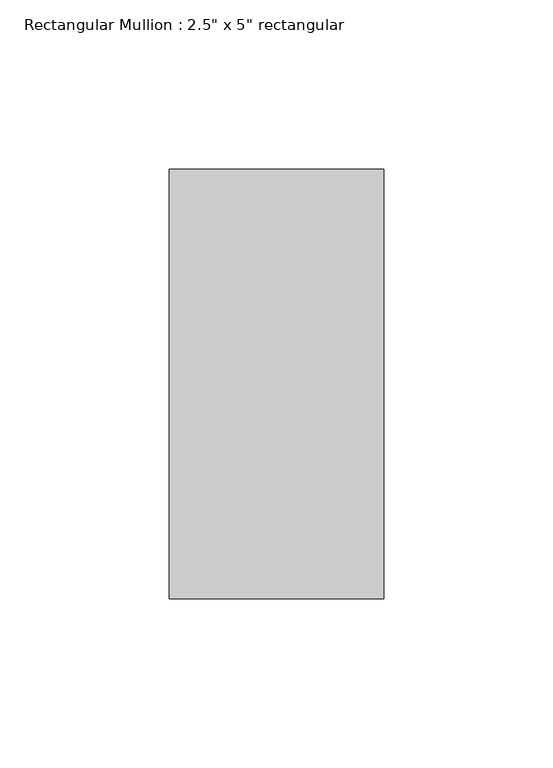
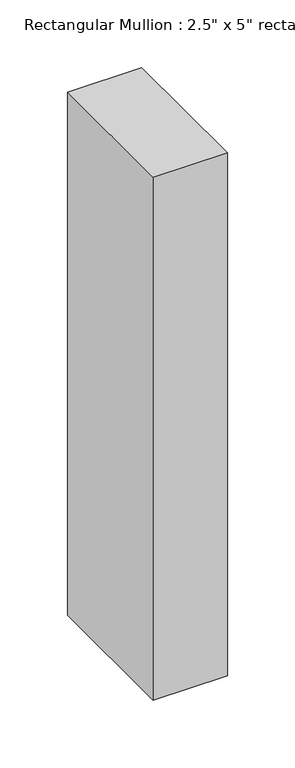
"""IFC4 building model written with IfcOpenShell, lengths in millimetres: member geometry."""

from ifc_helpers import new_model, si_unit, frame, origin, place, context, project, spatial, polyline, outline, extrude, source, transform, mapped, element, save


def member_e4ba5a11(model_context):
    return source(origin(), model_context, "Body", "SweptSolid", [
        extrude(outline(polyline([(0.0, 63.5), (0.0, -63.5), (-63.5, -63.5), (-63.5, 63.5), (0.0, 63.5)])), frame((0.0, 0.0, -472.45), z_axis=(0.0, 0.0, 1.0), x_axis=(1.0, 0.0, 0.0)), (0.0, 0.0, 1.0), 472.45),
    ])


if __name__ == "__main__":
    model = new_model("IFC4")
    model_context = context("Model", 3, world=origin())
    ifc_project = project(units=[si_unit("LENGTHUNIT", "METRE", prefix="MILLI")], contexts=[model_context])
    site = spatial("IfcSite", under=ifc_project)
    building = spatial("IfcBuilding", under=site)
    placement = place(None, origin())
    member_shape = member_e4ba5a11(model_context)
    element("IfcMember", 1, ObjectType="Rectangular Mullion : 2.5\" x 5\" rectangular", at=placement, inside=building, context=model_context, shape_type="MappedRepresentation", body=[
        mapped(member_shape, transform((0.0, 0.0, 0.0), x_axis=(1.0, 0.0, 0.0), y_axis=(0.0, 1.0, 0.0), z_axis=(0.0, 0.0, 1.0))),
    ])
    save(model, "model.ifc")

# Revit data of these elements
# Type "Rectangular Mullion : 2.5\" x 5\" rectangular"
#   built-in parameter 1007304 = 0.416667 (stored number, unit not read)
#   built-in parameter 1007301 = 0.104167 (stored number, unit not read)
#   built-in parameter 1007300 = 0.104167 (stored number, unit not read)
# Element 1 (IfcMember, "Rectangular Mullion : 2.5\" x 5\" rectangular")
#   Materials on its faces: "Damp-proofing"
# Materials
#   "Damp-proofing": class "Generic", colour RGB 127 127 127, transparency 0, Description = "Damp-proofing", Cost = 0
